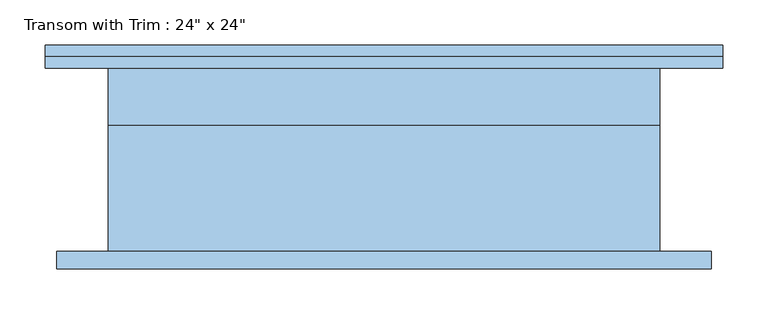
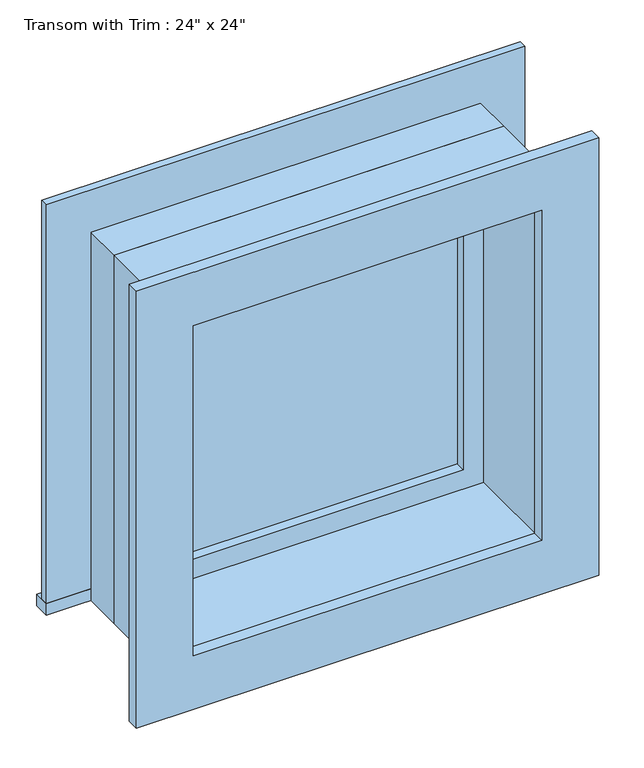
"""IFC4 building model written with IfcOpenShell, lengths in millimetres: window geometry."""

from ifc_helpers import new_model, si_unit, frame, origin, place, context, project, spatial, polyline, outline, extrude, source, transform, mapped, element, save


def window_e41d21a6(model_context):
    return source(origin(), model_context, "Body", "SweptSolid", [
        extrude(outline(polyline([(-412.75, 127.0), (336.55, 127.0), (336.55, 101.6), (-412.75, 101.6), (-412.75, 127.0)])), frame((0.0, 0.0, 2159.0), z_axis=(0.0, 0.0, 1.0), x_axis=(1.0, 0.0, 0.0)), (0.0, 0.0, 1.0), 19.05),
        extrude(outline(polyline([(2749.55, -323.85), (2749.55, 247.65), (2178.05, 247.65), (2178.05, 336.55), (2838.45, 336.55), (2838.45, -412.75), (2178.05, -412.75), (2178.05, -323.85), (2749.55, -323.85)])), frame((0.0, 101.6, 0.0), z_axis=(0.0, 1.0, 0.0), x_axis=(0.0, 0.0, 1.0)), (0.0, 0.0, 1.0), 12.7),
        extrude(outline(polyline([(2825.75, 323.85), (2825.75, -400.05), (2101.85, -400.05), (2101.85, 323.85), (2825.75, 323.85)]), holes=[polyline([(2736.85, 234.95), (2190.75, 234.95), (2190.75, -311.15), (2736.85, -311.15), (2736.85, 234.95)])]), frame((0.0, -120.65, 0.0), z_axis=(0.0, 1.0, 0.0), x_axis=(0.0, 0.0, 1.0)), (0.0, 0.0, 1.0), 19.05),
        extrude(outline(polyline([(203.2, 53.975), (-279.4, 53.975), (-279.4, 66.675), (203.2, 66.675), (203.2, 53.975)])), frame((0.0, 0.0, 2222.5), z_axis=(0.0, 0.0, 1.0), x_axis=(1.0, 0.0, 0.0)), (0.0, 0.0, 1.0), 482.6),
        extrude(outline(polyline([(2749.55, -323.85), (2178.05, -323.85), (2178.05, 247.65), (2749.55, 247.65), (2749.55, -323.85)]), holes=[polyline([(2705.1, -279.4), (2705.1, 203.2), (2222.5, 203.2), (2222.5, -279.4), (2705.1, -279.4)])]), frame((0.0, 38.1, 0.0), z_axis=(0.0, 1.0, 0.0), x_axis=(0.0, 0.0, 1.0)), (0.0, 0.0, 1.0), 44.45),
        extrude(outline(polyline([(2768.6, -342.9), (2159.0, -342.9), (2159.0, 266.7), (2768.6, 266.7), (2768.6, -342.9)]), holes=[polyline([(2736.85, -311.15), (2736.85, 234.95), (2190.75, 234.95), (2190.75, -311.15), (2736.85, -311.15)])]), frame((0.0, -101.6, 0.0), z_axis=(0.0, 1.0, 0.0), x_axis=(0.0, 0.0, 1.0)), (0.0, 0.0, 1.0), 139.7),
        extrude(outline(polyline([(2768.6, 266.7), (2768.6, -342.9), (2159.0, -342.9), (2159.0, 266.7), (2768.6, 266.7)]), holes=[polyline([(2749.55, 247.65), (2178.05, 247.65), (2178.05, -323.85), (2749.55, -323.85), (2749.55, 247.65)])]), frame((0.0, 38.1, 0.0), z_axis=(0.0, 1.0, 0.0), x_axis=(0.0, 0.0, 1.0)), (0.0, 0.0, 1.0), 63.5),
    ])


if __name__ == "__main__":
    model = new_model("IFC4")
    model_context = context("Model", 3, world=origin())
    ifc_project = project(units=[si_unit("LENGTHUNIT", "METRE", prefix="MILLI")], contexts=[model_context])
    site = spatial("IfcSite", under=ifc_project)
    building = spatial("IfcBuilding", under=site)
    placement = place(None, origin())
    window_shape = window_e41d21a6(model_context)
    element("IfcWindow", 1, ObjectType="Transom with Trim : 24\" x 24\"", at=placement, inside=building, context=model_context, shape_type="MappedRepresentation", body=[
        mapped(window_shape, transform((0.0, 0.0, 0.0), x_axis=(1.0, 0.0, 0.0), y_axis=(0.0, 1.0, 0.0), z_axis=(0.0, 0.0, 1.0))),
    ])
    save(model, "model.ifc")

# Revit data of these elements
# Type "Transom with Trim : 24\" x 24\""
#   Type Mark = "22"
#   Construction Type Id = "GSP4R"
#   Assembly Code = "B2020100"
#   Analytic Construction = "1/8 in Pilkington single glazing"
#   Visual Light Transmittance = 0.9
#   Solar Heat Gain Coefficient = 0.78
#   Heat Transfer Coefficient (U) = 0.6496 BTU/(h·ft²·°F)
#   Height = 2' - 0"
#   Default Sill Height = 7' - 1"
#   Trim Projection - Ext. = 0' - 0 1/2"
#   Trim Projection - Int. = 0' - 0 3/4"
#   Trim Width - Exterior = 0' - 3 1/2"
#   Trim Width - Interior = 0' - 3 1/2"
#   Width = 2' - 0"
#   Window Inset = 0' - 0 3/4"
#   Define Thermal Properties by = 1
#   Glass Pane Material = Glass
#   Sash Material = Sash
#   Trim Exterior Material = Trim
#   Trim Interior Material = Trim
#   Wall Closure = (empty or 0)
# Element 1 (IfcWindow, "Transom with Trim : 24\" x 24\"")
#   Materials on its faces: "Sash", "Trim", "Glass"
# Materials
#   "Glass": class "Glass", colour RGB 0 128 192, transparency 0.75, Description = "Soda Lime Glass", Cost = 0
#   "Sash": class "Wood", colour RGB 224 178 126, transparency 0
#   "Trim": class "Wood", colour RGB 224 178 126, transparency 0
